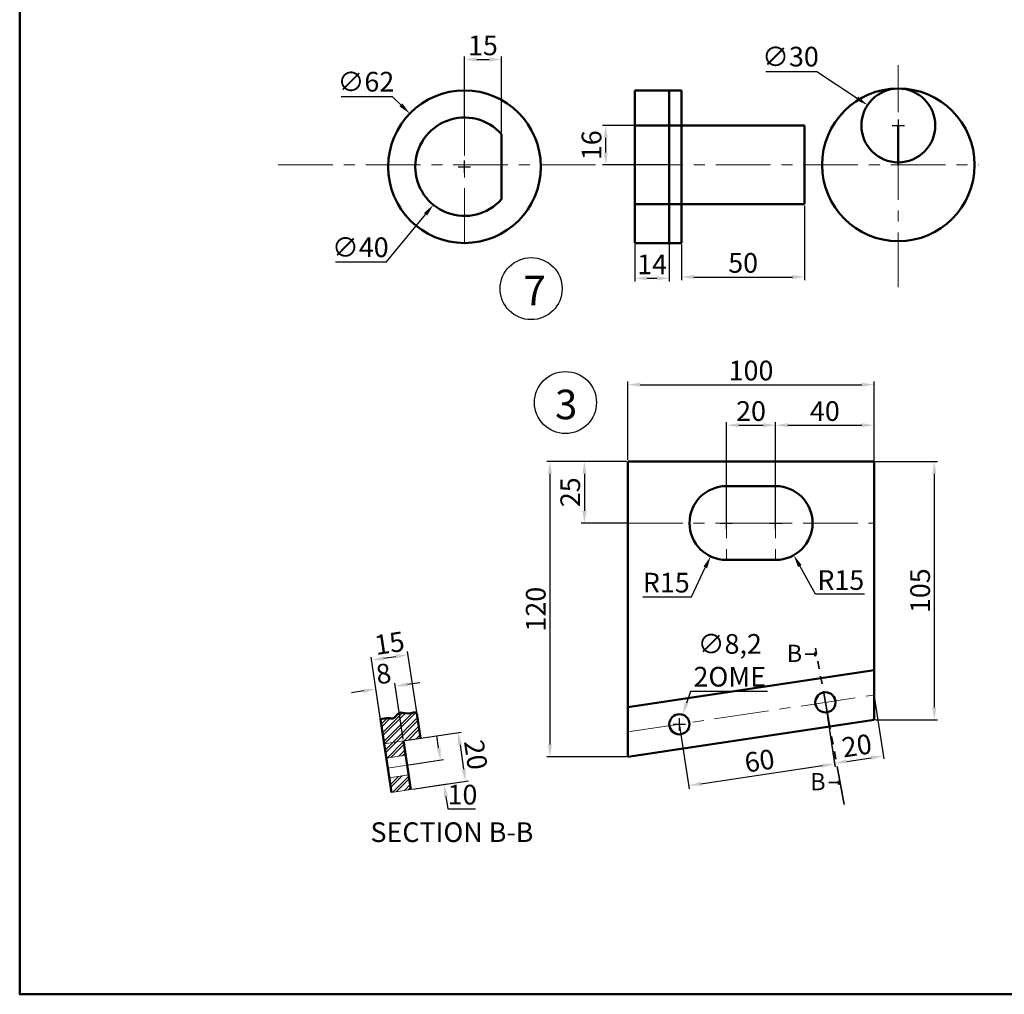
# Model space of a CAD drawing. Units: millimetres. Extents: x -749 to 333, y -22 to 680.
# Tile 1 of 4: x -749 to -349, y -22 to 374. Entities that reach past the tile are written whole.
import ezdxf

# ---------------------------------------------------------------- set-up
doc = ezdxf.new("R2010")
doc.units = ezdxf.units.MM
doc.header["$LTSCALE"] = 0.7
doc.linetypes.add('CENTER', pattern=[50.8, 31.75, -6.35, 6.35, -6.35])
doc.linetypes.add('PHANTOM', pattern=[63.5, 31.75, -6.35, 6.35, -6.35, 6.35, -6.35])
for name, color, linetype, lineweight in [('M-CNTR', 1, 'CENTER', 18), ('M-DIMS', 2, 'Continuous', 25), ('M-HATC', 8, 'Continuous', 18), ('M-OUTL', 7, 'Continuous', 50), ('M-SECT', 6, 'PHANTOM', 35), ('M-TEXT', 3, 'Continuous', 25), ('M-TTLB', 7, 'Continuous', 50)]:
    doc.layers.add(name, color=color, linetype=linetype, lineweight=lineweight)
doc.styles.get("Standard").update_dxf_attribs({"font": 'arial.ttf'})
doc.dimstyles.new('ISO-25', dxfattribs={"dimtxt": 8, "dimasz": 5, "dimexe": 1.25, "dimexo": 0.625, "dimtad": 1, "dimtoh": 1, "dimtxsty": 'Standard', "dimcen": 2.5, "dimadec": 0, "dimazin": 0, "dimtfac": 1, "dimtofl": 0, "dimtmove": 0, "dimatfit": 3, "dimfxl": 1, "dimarcsym": 0})

# ---------------------------------------------------------------- blocks, each defined once
blk = doc.blocks.new('*D36')
at = {"layer": 'Defpoints', "color": 0, "transparency": 16777216}
for p in [(-590.85, 335.54), (-546.39, 292.33)]:
    blk.add_point(p, dxfattribs=at)
at = {"layer": 'M-DIMS', "color": 0, "lineweight": -2, "transparency": 16777216}
for p, q in [((-618.72, 342.51), (-598.02, 342.51)), ((-598.02, 342.51), (-594.43, 339.03)), ((-568.62, 311.43), (-568.62, 316.43)), ((-571.12, 313.93), (-566.12, 313.93))]:
    blk.add_line(p, q, dxfattribs=at)
at = {"layer": 'M-DIMS', "color": 0, "transparency": 16777216}
blk.add_solid([(-593.85, 339.62), (-595.01, 338.43), (-590.85, 335.54)], dxfattribs=at)
at = {"layer": 'M-DIMS', "color": 0, "transparency": 16777216, "insert": (-608.68, 347.44), "char_height": 8, "attachment_point": 5}
blk.add_mtext('∅62', dxfattribs=at)
blk = doc.blocks.new('*D37')
at = {"layer": 'Defpoints', "color": 0, "transparency": 16777216}
for p in [(-555.96, 329.42), (-581.28, 298.45)]:
    blk.add_point(p, dxfattribs=at)
at = {"layer": 'M-DIMS', "color": 0, "lineweight": -2, "transparency": 16777216}
for p, q in [((-568.62, 311.43), (-568.62, 316.43)), ((-571.12, 313.93), (-566.12, 313.93)), ((-600.26, 275.24), (-584.44, 294.58)), ((-621.02, 275.24), (-600.26, 275.24))]:
    blk.add_line(p, q, dxfattribs=at)
at = {"layer": 'M-DIMS', "color": 0, "transparency": 16777216}
blk.add_solid([(-585.09, 295.11), (-583.79, 294.05), (-581.28, 298.45)], dxfattribs=at)
at = {"layer": 'M-DIMS', "color": 0, "transparency": 16777216, "insert": (-610.95, 280.17), "char_height": 8, "attachment_point": 5}
blk.add_mtext('∅40', dxfattribs=at)
blk = doc.blocks.new('*D38')
at = {"layer": 'Defpoints', "color": 0, "transparency": 16777216}
for p in [(-404.82, 338.98), (-379.83, 322.39)]:
    blk.add_point(p, dxfattribs=at)
at = {"layer": 'M-DIMS', "color": 0, "lineweight": -2, "transparency": 16777216}
for p, q in [((-446.23, 352.68), (-425.47, 352.68)), ((-425.47, 352.68), (-408.99, 341.74)), ((-392.32, 328.18), (-392.32, 333.18)), ((-394.82, 330.68), (-389.82, 330.68))]:
    blk.add_line(p, q, dxfattribs=at)
at = {"layer": 'M-DIMS', "color": 0, "transparency": 16777216}
blk.add_solid([(-408.53, 342.44), (-409.45, 341.05), (-404.82, 338.98)], dxfattribs=at)
at = {"layer": 'M-DIMS', "color": 0, "transparency": 16777216, "insert": (-436.16, 357.62), "char_height": 8, "attachment_point": 5}
blk.add_mtext('∅30', dxfattribs=at)
blk = doc.blocks.new('*D39')
at = {"layer": 'Defpoints', "color": 0, "transparency": 16777216}
for p in [(-511.24, 330.68), (-485.39, 330.68), (-485.39, 314.68)]:
    blk.add_point(p, dxfattribs=at)
at = {"layer": 'M-DIMS', "color": 0, "lineweight": -2, "transparency": 16777216}
for p, q in [((-486.01, 330.68), (-512.49, 330.68)), ((-511.24, 319.68), (-511.24, 325.68)), ((-486.01, 314.68), (-512.49, 314.68))]:
    blk.add_line(p, q, dxfattribs=at)
at = {"layer": 'M-DIMS', "color": 0, "transparency": 16777216}
for points in [[(-512.07, 325.68), (-510.4, 325.68), (-511.24, 330.68)], [(-512.07, 319.68), (-510.4, 319.68), (-511.24, 314.68)]]:
    blk.add_solid(points, dxfattribs=at)
at = {"layer": 'M-DIMS', "color": 0, "transparency": 16777216, "insert": (-515.95, 322.68), "char_height": 8, "attachment_point": 5, "rotation": 90}
blk.add_mtext('16', dxfattribs=at)
blk = doc.blocks.new('*D40')
at = {"layer": 'Defpoints', "color": 0, "transparency": 16777216}
for p in [(-499.39, 282.93), (-485.39, 282.93), (-485.39, 268.59)]:
    blk.add_point(p, dxfattribs=at)
at = {"layer": 'M-DIMS', "color": 0, "lineweight": -2, "transparency": 16777216}
for p, q in [((-499.39, 282.31), (-499.39, 267.34)), ((-485.39, 282.31), (-485.39, 267.34)), ((-494.39, 268.59), (-490.39, 268.59))]:
    blk.add_line(p, q, dxfattribs=at)
at = {"layer": 'M-DIMS', "color": 0, "transparency": 16777216}
for points in [[(-494.39, 269.42), (-494.39, 267.76), (-499.39, 268.59)], [(-490.39, 269.42), (-490.39, 267.76), (-485.39, 268.59)]]:
    blk.add_solid(points, dxfattribs=at)
at = {"layer": 'M-DIMS', "color": 0, "transparency": 16777216, "insert": (-492.39, 273.23), "char_height": 8, "attachment_point": 5}
blk.add_mtext('14', dxfattribs=at)
blk = doc.blocks.new('*D41')
at = {"layer": 'Defpoints', "color": 0, "transparency": 16777216}
for p in [(-430.39, 298.68), (-480.39, 282.93), (-430.39, 269.12)]:
    blk.add_point(p, dxfattribs=at)
at = {"layer": 'M-DIMS', "color": 0, "lineweight": -2, "transparency": 16777216}
for p, q in [((-430.39, 298.06), (-430.39, 267.87)), ((-480.39, 282.31), (-480.39, 267.87)), ((-475.39, 269.12), (-435.39, 269.12))]:
    blk.add_line(p, q, dxfattribs=at)
at = {"layer": 'M-DIMS', "color": 0, "transparency": 16777216}
for points in [[(-475.39, 269.95), (-475.39, 268.29), (-480.39, 269.12)], [(-435.39, 269.95), (-435.39, 268.29), (-430.39, 269.12)]]:
    blk.add_solid(points, dxfattribs=at)
at = {"layer": 'M-DIMS', "color": 0, "transparency": 16777216, "insert": (-455.39, 273.83), "char_height": 8, "attachment_point": 5}
blk.add_mtext('50', dxfattribs=at)
blk = doc.blocks.new('*D42')
at = {"layer": 'Defpoints', "color": 0, "transparency": 16777216}
for p in [(-553.62, 357.49), (-568.62, 333.93), (-553.62, 327.16)]:
    blk.add_point(p, dxfattribs=at)
at = {"layer": 'M-DIMS', "color": 0, "lineweight": -2, "transparency": 16777216}
for p, q in [((-568.62, 334.56), (-568.62, 358.74)), ((-563.62, 357.49), (-558.62, 357.49)), ((-553.62, 327.79), (-553.62, 358.74))]:
    blk.add_line(p, q, dxfattribs=at)
at = {"layer": 'M-DIMS', "color": 0, "transparency": 16777216}
for points in [[(-563.62, 358.32), (-563.62, 356.65), (-568.62, 357.49)], [(-558.62, 358.32), (-558.62, 356.65), (-553.62, 357.49)]]:
    blk.add_solid(points, dxfattribs=at)
at = {"layer": 'M-DIMS', "color": 0, "transparency": 16777216, "insert": (-561.12, 362.19), "char_height": 8, "attachment_point": 5}
blk.add_mtext('15', dxfattribs=at)
blk = doc.blocks.new('*D66')
at = {"layer": 'Defpoints', "color": 0, "transparency": 16777216}
for p in [(-402.18, 225.38), (-502.18, 194.18), (-402.18, 194.18)]:
    blk.add_point(p, dxfattribs=at)
at = {"layer": 'M-DIMS', "color": 0, "lineweight": -2, "transparency": 16777216}
for p, q in [((-502.18, 194.8), (-502.18, 226.63)), ((-497.18, 225.38), (-407.18, 225.38)), ((-402.18, 194.8), (-402.18, 226.63))]:
    blk.add_line(p, q, dxfattribs=at)
at = {"layer": 'M-DIMS', "color": 0, "transparency": 16777216}
for points in [[(-497.18, 226.22), (-497.18, 224.55), (-502.18, 225.38)], [(-407.18, 226.22), (-407.18, 224.55), (-402.18, 225.38)]]:
    blk.add_solid(points, dxfattribs=at)
at = {"layer": 'M-DIMS', "color": 0, "transparency": 16777216, "insert": (-452.18, 230.09), "char_height": 8, "attachment_point": 5}
blk.add_mtext('100', dxfattribs=at)
blk = doc.blocks.new('*D67')
at = {"layer": 'Defpoints', "color": 0, "transparency": 16777216}
for p in [(-402.18, 194.18), (-402.18, 89.18), (-377.71, 89.18)]:
    blk.add_point(p, dxfattribs=at)
at = {"layer": 'M-DIMS', "color": 0, "lineweight": -2, "transparency": 16777216}
for p, q in [((-401.55, 194.18), (-376.46, 194.18)), ((-377.71, 189.18), (-377.71, 94.18)), ((-401.55, 89.18), (-376.46, 89.18))]:
    blk.add_line(p, q, dxfattribs=at)
at = {"layer": 'M-DIMS', "color": 0, "transparency": 16777216}
for points in [[(-378.54, 189.18), (-376.87, 189.18), (-377.71, 194.18)], [(-378.54, 94.18), (-376.87, 94.18), (-377.71, 89.18)]]:
    blk.add_solid(points, dxfattribs=at)
at = {"layer": 'M-DIMS', "color": 0, "transparency": 16777216, "insert": (-382.42, 141.68), "char_height": 8, "attachment_point": 5, "rotation": 90}
blk.add_mtext('105', dxfattribs=at)
blk = doc.blocks.new('*D68')
at = {"layer": 'Defpoints', "color": 0, "transparency": 16777216}
for p in [(-442.18, 208.92), (-462.18, 169.18), (-442.18, 169.18)]:
    blk.add_point(p, dxfattribs=at)
at = {"layer": 'M-DIMS', "color": 0, "lineweight": -2, "transparency": 16777216}
for p, q in [((-462.18, 169.8), (-462.18, 210.17)), ((-457.18, 208.92), (-447.18, 208.92)), ((-442.18, 169.8), (-442.18, 210.17))]:
    blk.add_line(p, q, dxfattribs=at)
at = {"layer": 'M-DIMS', "color": 0, "transparency": 16777216}
for points in [[(-457.18, 209.75), (-457.18, 208.08), (-462.18, 208.92)], [(-447.18, 209.75), (-447.18, 208.08), (-442.18, 208.92)]]:
    blk.add_solid(points, dxfattribs=at)
at = {"layer": 'M-DIMS', "color": 0, "transparency": 16777216, "insert": (-452.18, 213.63), "char_height": 8, "attachment_point": 5}
blk.add_mtext('20', dxfattribs=at)
blk = doc.blocks.new('*D69')
at = {"layer": 'Defpoints', "color": 0, "transparency": 16777216}
for p in [(-502.18, 194.18), (-519.89, 169.18), (-502.18, 169.18)]:
    blk.add_point(p, dxfattribs=at)
at = {"layer": 'M-DIMS', "color": 0, "lineweight": -2, "transparency": 16777216}
for p, q in [((-502.8, 194.18), (-521.14, 194.18)), ((-519.89, 189.18), (-519.89, 174.18)), ((-502.8, 169.18), (-521.14, 169.18))]:
    blk.add_line(p, q, dxfattribs=at)
at = {"layer": 'M-DIMS', "color": 0, "transparency": 16777216}
for points in [[(-520.72, 189.18), (-519.05, 189.18), (-519.89, 194.18)], [(-520.72, 174.18), (-519.05, 174.18), (-519.89, 169.18)]]:
    blk.add_solid(points, dxfattribs=at)
at = {"layer": 'M-DIMS', "color": 0, "transparency": 16777216, "insert": (-524.6, 181.68), "char_height": 8, "attachment_point": 5, "rotation": 90}
blk.add_mtext('25', dxfattribs=at)
blk = doc.blocks.new('*D70')
at = {"layer": 'Defpoints', "color": 0, "transparency": 16777216}
for p in [(-421.96, 96.32), (-481.29, 87.42), (-418.21, 71.38)]:
    blk.add_point(p, dxfattribs=at)
at = {"layer": 'M-DIMS', "color": 0, "lineweight": -2, "transparency": 16777216}
for p, q in [((-421.86, 95.7), (-418.03, 70.14)), ((-481.2, 86.8), (-477.37, 61.24)), ((-472.61, 63.22), (-423.16, 70.64))]:
    blk.add_line(p, q, dxfattribs=at)
at = {"layer": 'M-DIMS', "color": 0, "transparency": 16777216}
for points in [[(-423.28, 71.46), (-423.04, 69.81), (-418.21, 71.38)], [(-472.73, 64.04), (-472.48, 62.39), (-477.55, 62.48)]]:
    blk.add_solid(points, dxfattribs=at)
at = {"layer": 'M-DIMS', "color": 0, "transparency": 16777216, "insert": (-448.58, 71.58), "char_height": 8, "attachment_point": 5, "rotation": 8.5308}
blk.add_mtext('60', dxfattribs=at)
blk = doc.blocks.new('*D71')
at = {"layer": 'Defpoints', "color": 0, "transparency": 16777216}
for p in [(-421.96, 96.32), (-402.18, 99.29), (-398.47, 74.54)]:
    blk.add_point(p, dxfattribs=at)
at = {"layer": 'M-DIMS', "color": 0, "lineweight": -2, "transparency": 16777216}
for p, q in [((-402.08, 98.67), (-398.28, 73.31)), ((-421.86, 95.7), (-418.06, 70.34)), ((-413.3, 72.32), (-403.41, 73.8))]:
    blk.add_line(p, q, dxfattribs=at)
at = {"layer": 'M-DIMS', "color": 0, "transparency": 16777216}
for points in [[(-413.42, 73.14), (-413.18, 71.49), (-418.24, 71.57)], [(-403.53, 74.62), (-403.29, 72.98), (-398.47, 74.54)]]:
    blk.add_solid(points, dxfattribs=at)
at = {"layer": 'M-DIMS', "color": 0, "transparency": 16777216, "insert": (-409.05, 77.72), "char_height": 8, "attachment_point": 5, "rotation": 8.5308}
blk.add_mtext('20', dxfattribs=at)
blk = doc.blocks.new('*D72')
at = {"layer": 'Defpoints', "color": 0, "transparency": 16777216}
for p in [(-502.18, 194.18), (-533.91, 74.18), (-502.18, 74.18)]:
    blk.add_point(p, dxfattribs=at)
at = {"layer": 'M-DIMS', "color": 0, "lineweight": -2, "transparency": 16777216}
for p, q in [((-502.8, 194.18), (-535.16, 194.18)), ((-533.91, 189.18), (-533.91, 79.18)), ((-502.8, 74.18), (-535.16, 74.18))]:
    blk.add_line(p, q, dxfattribs=at)
at = {"layer": 'M-DIMS', "color": 0, "transparency": 16777216}
for points in [[(-534.75, 189.18), (-533.08, 189.18), (-533.91, 194.18)], [(-534.75, 79.18), (-533.08, 79.18), (-533.91, 74.18)]]:
    blk.add_solid(points, dxfattribs=at)
at = {"layer": 'M-DIMS', "color": 0, "transparency": 16777216, "insert": (-538.62, 134.18), "char_height": 8, "attachment_point": 5, "rotation": 90}
blk.add_mtext('120', dxfattribs=at)
blk = doc.blocks.new('*D73')
at = {"layer": 'Defpoints', "color": 0, "transparency": 16777216}
for p in [(-479.99, 91.31), (-482.59, 83.53)]:
    blk.add_point(p, dxfattribs=at)
at = {"layer": 'M-DIMS', "color": 0, "lineweight": -2, "transparency": 16777216}
for p, q in [((-476.81, 100.79), (-478.4, 96.05)), ((-445.44, 100.79), (-476.81, 100.79)), ((-481.29, 84.92), (-481.29, 89.92)), ((-483.79, 87.42), (-478.79, 87.42))]:
    blk.add_line(p, q, dxfattribs=at)
at = {"layer": 'M-DIMS', "color": 0, "transparency": 16777216}
blk.add_solid([(-479.19, 96.31), (-477.61, 95.78), (-479.99, 91.31)], dxfattribs=at)
at = {"layer": 'M-DIMS', "color": 0, "transparency": 16777216, "insert": (-460.82, 112.37), "char_height": 8, "attachment_point": 5}
blk.add_mtext('∅8,2\\P2OME', dxfattribs=at)
blk = doc.blocks.new('*D74')
at = {"layer": 'Defpoints', "color": 0, "transparency": 16777216}
for p in [(-462.18, 169.18), (-468.61, 155.63)]:
    blk.add_point(p, dxfattribs=at)
at = {"layer": 'M-DIMS', "color": 0, "lineweight": -2, "transparency": 16777216}
for p, q in [((-464.68, 169.18), (-459.68, 169.18)), ((-462.18, 166.68), (-462.18, 171.68)), ((-476.41, 139.22), (-470.76, 151.11)), ((-496.21, 139.22), (-476.41, 139.22))]:
    blk.add_line(p, q, dxfattribs=at)
at = {"layer": 'M-DIMS', "color": 0, "transparency": 16777216}
blk.add_solid([(-471.51, 151.47), (-470.01, 150.75), (-468.61, 155.63)], dxfattribs=at)
at = {"layer": 'M-DIMS', "color": 0, "transparency": 16777216, "insert": (-486.62, 143.92), "char_height": 8, "attachment_point": 5}
blk.add_mtext('R15', dxfattribs=at)
blk = doc.blocks.new('*D75')
at = {"layer": 'Defpoints', "color": 0, "transparency": 16777216}
for p in [(-442.18, 169.18), (-434.83, 156.1)]:
    blk.add_point(p, dxfattribs=at)
at = {"layer": 'M-DIMS', "color": 0, "lineweight": -2, "transparency": 16777216}
for p, q in [((-444.68, 169.18), (-439.68, 169.18)), ((-442.18, 166.68), (-442.18, 171.68)), ((-425.92, 140.26), (-432.38, 151.74)), ((-406.12, 140.26), (-425.92, 140.26))]:
    blk.add_line(p, q, dxfattribs=at)
at = {"layer": 'M-DIMS', "color": 0, "transparency": 16777216}
blk.add_solid([(-431.65, 152.15), (-433.1, 151.33), (-434.83, 156.1)], dxfattribs=at)
at = {"layer": 'M-DIMS', "color": 0, "transparency": 16777216, "insert": (-415.71, 144.97), "char_height": 8, "attachment_point": 5}
blk.add_mtext('R15', dxfattribs=at)
blk = doc.blocks.new('*D76')
at = {"layer": 'Defpoints', "color": 0, "transparency": 16777216}
for p in [(-593.38, 80.72), (-568.22, 64.27), (-590.41, 60.94)]:
    blk.add_point(p, dxfattribs=at)
at = {"layer": 'M-DIMS', "color": 0, "lineweight": -2, "transparency": 16777216}
for p, q in [((-592.76, 80.81), (-569.95, 84.23)), ((-570.44, 79.1), (-568.96, 69.22)), ((-589.79, 61.03), (-566.98, 64.46))]:
    blk.add_line(p, q, dxfattribs=at)
at = {"layer": 'M-DIMS', "color": 0, "transparency": 16777216}
for points in [[(-569.62, 79.23), (-571.27, 78.98), (-571.18, 84.05)], [(-568.13, 69.34), (-569.78, 69.09), (-568.22, 64.27)]]:
    blk.add_solid(points, dxfattribs=at)
at = {"layer": 'M-DIMS', "color": 0, "transparency": 16777216, "insert": (-565.04, 74.86), "char_height": 8, "attachment_point": 5, "rotation": 278.5308}
blk.add_mtext('20', dxfattribs=at)
blk = doc.blocks.new('*D77')
at = {"layer": 'Defpoints', "color": 0, "transparency": 16777216}
for p in [(-591.89, 70.83), (-590.41, 60.94), (-576.89, 62.97)]:
    blk.add_point(p, dxfattribs=at)
at = {"layer": 'M-DIMS', "color": 0, "lineweight": -2, "transparency": 16777216}
for p, q in [((-579.11, 77.8), (-579.85, 82.75)), ((-591.28, 70.92), (-577.13, 73.04)), ((-589.79, 61.03), (-575.65, 63.16)), ((-576.15, 58.03), (-575.4, 53.08)), ((-575.4, 53.08), (-564.1, 53.08))]:
    blk.add_line(p, q, dxfattribs=at)
at = {"layer": 'M-DIMS', "color": 0, "transparency": 16777216}
for points in [[(-578.29, 77.93), (-579.94, 77.68), (-578.37, 72.86)], [(-575.32, 58.15), (-576.97, 57.9), (-576.89, 62.97)]]:
    blk.add_solid(points, dxfattribs=at)
at = {"layer": 'M-DIMS', "color": 0, "transparency": 16777216, "insert": (-569.44, 57.79), "char_height": 8, "attachment_point": 5}
blk.add_mtext('10', dxfattribs=at)
blk = doc.blocks.new('*D78')
at = {"layer": 'Defpoints', "color": 0, "transparency": 16777216}
for p in [(-591.55, 115.71), (-602.77, 89.44), (-587.94, 91.66)]:
    blk.add_point(p, dxfattribs=at)
at = {"layer": 'M-DIMS', "color": 0, "lineweight": -2, "transparency": 16777216}
for p, q in [((-588.03, 92.28), (-591.73, 116.95)), ((-602.87, 90.06), (-606.57, 114.72)), ((-601.44, 114.23), (-596.49, 114.97))]:
    blk.add_line(p, q, dxfattribs=at)
at = {"layer": 'M-DIMS', "color": 0, "transparency": 16777216}
for points in [[(-601.56, 115.05), (-601.31, 113.4), (-606.38, 113.49)], [(-596.62, 115.79), (-596.37, 114.15), (-591.55, 115.71)]]:
    blk.add_solid(points, dxfattribs=at)
at = {"layer": 'M-DIMS', "color": 0, "transparency": 16777216, "insert": (-598.95, 119.36), "char_height": 8, "attachment_point": 5, "rotation": 8.5308}
blk.add_mtext('15', dxfattribs=at)
blk = doc.blocks.new('*D79')
at = {"layer": 'Defpoints', "color": 0, "transparency": 16777216}
for p in [(-596.71, 102.91), (-593.38, 80.72), (-601.29, 79.53)]:
    blk.add_point(p, dxfattribs=at)
at = {"layer": 'M-DIMS', "color": 0, "lineweight": -2, "transparency": 16777216}
for p, q in [((-593.47, 81.34), (-596.89, 104.14)), ((-591.76, 103.65), (-586.82, 104.39)), ((-609.56, 100.98), (-614.51, 100.24)), ((-601.38, 80.15), (-604.8, 102.96))]:
    blk.add_line(p, q, dxfattribs=at)
at = {"layer": 'M-DIMS', "color": 0, "transparency": 16777216}
for points in [[(-591.88, 104.47), (-591.64, 102.83), (-596.71, 102.91)], [(-609.69, 101.8), (-609.44, 100.16), (-604.62, 101.72)]]:
    blk.add_solid(points, dxfattribs=at)
at = {"layer": 'M-DIMS', "color": 0, "transparency": 16777216, "insert": (-601.36, 106.97), "char_height": 8, "attachment_point": 5, "rotation": 8.5308}
blk.add_mtext('8', dxfattribs=at)
blk = doc.blocks.new('*D88')
at = {"layer": 'Defpoints', "color": 0, "ltscale": 0.7, "transparency": 16777216}
for p in [(-402.18, 208.92), (-402.18, 178.12), (-442.18, 169.18)]:
    blk.add_point(p, dxfattribs=at)
at = {"layer": 'M-DIMS', "color": 0, "lineweight": -2, "ltscale": 0.7, "transparency": 16777216}
for p, q in [((-442.18, 169.8), (-442.18, 210.17)), ((-437.18, 208.92), (-407.18, 208.92)), ((-402.18, 178.75), (-402.18, 210.17))]:
    blk.add_line(p, q, dxfattribs=at)
at = {"layer": 'M-DIMS', "color": 0, "ltscale": 0.7, "transparency": 16777216}
for points in [[(-437.18, 209.75), (-437.18, 208.08), (-442.18, 208.92)], [(-407.18, 209.75), (-407.18, 208.08), (-402.18, 208.92)]]:
    blk.add_solid(points, dxfattribs=at)
at = {"layer": 'M-DIMS', "color": 0, "ltscale": 0.7, "transparency": 16777216, "insert": (-422.18, 213.63), "char_height": 8, "attachment_point": 5}
blk.add_mtext('40', dxfattribs=at)

msp = doc.modelspace()

# ---------------------------------------------------------------- hatches: boundary and pattern name
at = {"layer": 'M-HATC', "ltscale": 0.7}
h = msp.add_hatch(dxfattribs=at)
h.set_pattern_fill('ANSI32', color=256, scale=0.3)
h.set_pattern_definition([(45, (-3477.0897, -507.9452), (-2.0205576, 2.0205576), []), (45, (-3475.7427, -507.9452), (-2.0205576, 2.0205576), [])])
edge = h.paths.add_edge_path()
edge.add_spline(control_points=[(-587.97, 91.861), (-588.348, 92.607), (-591.937, 91.134), (-595.435, 93.056), (-597.003, 89.411), (-599.981, 90.2), (-601.71, 89.728), (-602.775, 89.438)], knot_values=[0, 0, 0, 0, 3.4976081, 7.5126071, 10.2409894, 12.3136778, 15.6403307, 15.6403307, 15.6403307, 15.6403307], degree=3, periodic=0)
edge.add_line((-602.775, 89.438), (-601.289, 79.533))
edge.add_line((-601.289, 79.533), (-586.455, 81.759))
edge.add_line((-586.455, 81.759), (-587.97, 91.861))
h.paths.add_polyline_path([(-593.378, 80.72), (-601.289, 79.533), (-600.408, 73.657), (-592.496, 74.844)])
h.paths.add_polyline_path([(-591.293, 66.823), (-599.205, 65.637), (-598.322, 59.755), (-590.411, 60.941)])

# ---------------------------------------------------------------- linework, layer by layer
at = {"layer": 'M-CNTR'}
for p, q in [((-392.323, 264.979), (-392.323, 355.252)), ((-568.616, 282.934), (-568.616, 344.934)), ((-644.284, 314.684), (-537.625, 314.684)), ((-537.625, 314.684), (-359.786, 314.684)), ((-462.178, 194.176), (-462.178, 154.176)), ((-442.178, 194.176), (-442.178, 154.176)), ((-502.178, 169.176), (-402.178, 169.176)), ((-502.178, 84.288), (-402.178, 99.288)), ((-402.178, 89.176), (-400.694, 89.399)), ((-601.289, 79.533), (-586.455, 81.759)), ((-600.408, 73.657), (-592.496, 74.844)), ((-599.806, 69.644), (-584.972, 71.869)), ((-599.205, 65.637), (-591.293, 66.823)), ((-598.322, 59.755), (-590.411, 60.941))]:
    msp.add_line(p, q, dxfattribs=at)
at = {"layer": 'M-OUTL'}
for p, q in [((-499.387, 282.934), (-499.387, 344.934)), ((-499.387, 344.934), (-485.387, 344.934)), ((-485.387, 344.934), (-485.387, 282.934)), ((-480.387, 344.934), (-485.387, 344.934)), ((-480.387, 344.934), (-480.387, 282.934)), ((-499.387, 330.684), (-430.387, 330.684)), ((-430.387, 298.684), (-430.387, 330.684)), ((-553.617, 300.703), (-553.617, 327.164)), ((-499.387, 298.684), (-430.387, 298.684)), ((-485.387, 282.934), (-499.387, 282.934)), ((-499.387, 282.934), (-480.387, 282.934)), ((-502.178, 194.176), (-402.178, 194.176)), ((-502.178, 194.176), (-502.178, 74.176)), ((-402.178, 194.176), (-402.178, 89.176)), ((-462.178, 184.176), (-442.178, 184.176)), ((-462.178, 154.176), (-442.178, 154.176)), ((-502.178, 94.4), (-402.178, 109.4)), ((-601.289, 79.533), (-602.775, 89.438)), ((-586.455, 81.759), (-587.97, 91.861)), ((-502.178, 74.176), (-402.178, 89.176)), ((-593.378, 80.72), (-590.411, 60.941)), ((-601.289, 79.533), (-598.322, 59.755))]:
    msp.add_line(p, q, dxfattribs=at)
at = {"layer": 'M-OUTL', "ltscale": 0.7}
msp.add_line((-392.323, 314.684), (-392.323, 330.684), dxfattribs=at)
at = {"layer": 'M-OUTL'}
for centre, radius in [((-568.616, 313.934), 31), ((-392.323, 314.684), 31), ((-392.323, 330.684), 15), ((-421.956, 96.321), 4.1), ((-481.292, 87.421), 4.1), ((-481.292, 87.421), 4.1)]:
    msp.add_circle(centre, radius, dxfattribs=at)
for centre, radius, start, end in [((-568.616, 313.934), 20, 41.41641, 318.58359), ((-462.178, 169.176), 15, 90, 270), ((-442.178, 169.176), 15, 270, 90)]:
    msp.add_arc(centre, radius, start, end, dxfattribs=at)
msp.add_open_spline([(-602.775, 89.438), (-601.71, 89.728), (-599.981, 90.2), (-597.003, 89.411), (-595.435, 93.056), (-591.937, 91.134), (-588.348, 92.607), (-587.97, 91.861)], degree=3, knots=[0, 0, 0, 0, 3.3266529, 5.3993413, 8.1277235, 12.1427226, 15.6403307, 15.6403307, 15.6403307, 15.6403307], dxfattribs=at)
at = {"layer": 'M-SECT', "ltscale": 0.7}
for p, q in [((-425.526, 115.851), (-426.233, 116.558)), ((-426.233, 116.558), (-426.233, 115.144)), ((-414.383, 54.891), (-425.971, 118.286)), ((-430.118, 115.853), (-425.526, 115.851)), ((-425.526, 115.851), (-426.233, 115.144)), ((-415.995, 63.711), (-416.702, 64.418)), ((-416.702, 64.418), (-416.702, 63.004)), ((-420.588, 63.713), (-415.995, 63.711)), ((-415.995, 63.711), (-416.702, 63.004))]:
    msp.add_line(p, q, dxfattribs=at)
at = {"layer": 'M-TEXT'}
for centre in [(-541.538, 264.395), (-527.586, 218.129)]:
    msp.add_circle(centre, 12.598, dxfattribs=at)
at = {"layer": 'M-TTLB', "ltscale": 0.7}
msp.add_lwpolyline([(-749.362, 679.91), (332.782, 679.91), (332.782, -22.287), (-749.362, -22.287)], close=True, dxfattribs=at)

# ---------------------------------------------------------------- texts
at = {"layer": 'M-TEXT', "attachment_point": 1}
for s, width, insert, char_height in [('7', 30.10277, (-544.685, 269.614), 12), ('\\pxql;3', 12, (-531.84, 223.348), 12), ('SECTION B-B', 95.89335, (-606.818, 47.575), 8)]:
    msp.add_mtext_dynamic_manual_height_columns(s, width=width, gutter_width=12.5, heights=[0], dxfattribs=dict(at, insert=insert, char_height=char_height))
at = {"layer": 'M-TEXT', "ltscale": 0.7, "char_height": 7, "attachment_point": 1}
for insert in [(-437.678, 119.727), (-428.148, 67.587)]:
    msp.add_mtext_dynamic_manual_height_columns('B', width=7.19522, gutter_width=12.5, heights=[0], dxfattribs=dict(at, insert=insert))

# ---------------------------------------------------------------- dimensions: what is measured, and where the dimension line sits
at = {"layer": 'M-DIMS'}
for base, p1, p2, picture, middle in [((-553.617, 357.485), (-568.616, 333.934), (-553.617, 327.164), '*D42', (-561.117, 362.195)), ((-430.387, 269.121), (-480.387, 282.934), (-430.387, 298.684), '*D41', (-455.387, 273.831)), ((-485.387, 268.591), (-499.387, 282.934), (-485.387, 282.934), '*D40', (-492.387, 273.232)), ((-402.178, 225.383), (-502.178, 194.176), (-402.178, 194.176), '*D66', (-452.178, 230.093)), ((-442.178, 208.916), (-462.178, 169.176), (-442.178, 169.176), '*D68', (-452.178, 213.626))]:
    dim = msp.add_linear_dim(base=base, p1=p1, p2=p2, dimstyle='ISO-25', override={"dimclrd": 0, "dimclre": 0, "dimclrt": 0}, dxfattribs=at)
    dim.commit()
    dim.dimension.update_dxf_attribs({"geometry": picture, "text_midpoint": middle})
for p1, p2, picture, middle in [((-379.825, 322.389), (-404.821, 338.979), '*D38', (-436.161, 352.683)), ((-555.956, 329.417), (-581.275, 298.45), '*D37', (-610.949, 275.235))]:
    dim = msp.add_diameter_dim_2p(p1=p1, p2=p2, dimstyle='ISO-25', override={"dimclrd": 0, "dimclre": 0, "dimclrt": 0}, dxfattribs=at)
    dim.commit()
    dim.dimension.update_dxf_attribs({"geometry": picture, "text_midpoint": middle, "dimtype": 163})
dim = msp.add_diameter_dim_2p(p1=(-546.386, 292.328), p2=(-590.846, 335.54), dimstyle='ISO-25', override={"dimclrd": 0, "dimclre": 0, "dimclrt": 0}, dxfattribs=at)
dim.commit()
dim.dimension.update_dxf_attribs({"geometry": '*D36', "text_midpoint": (-608.682, 347.443)})
for base, p1, p2, picture, middle in [((-511.237, 330.684), (-485.387, 314.684), (-485.387, 330.684), '*D39', (-515.947, 322.684)), ((-533.915, 74.176), (-502.178, 194.176), (-502.178, 74.176), '*D72', (-538.624, 134.176)), ((-519.887, 169.176), (-502.178, 194.176), (-502.178, 169.176), '*D69', (-524.596, 181.676)), ((-377.706, 89.176), (-402.178, 194.176), (-402.178, 89.176), '*D67', (-382.415, 141.676))]:
    dim = msp.add_linear_dim(base=base, p1=p1, p2=p2, angle=90, dimstyle='ISO-25', override={"dimclrd": 0, "dimclre": 0, "dimclrt": 0}, dxfattribs=at)
    dim.commit()
    dim.dimension.update_dxf_attribs({"geometry": picture, "text_midpoint": middle})
at = {"layer": 'M-DIMS', "ltscale": 0.7}
dim = msp.add_linear_dim(base=(-402.178, 208.916), p1=(-442.178, 169.176), p2=(-402.178, 178.122), dimstyle='ISO-25', override={"dimclrd": 0, "dimclre": 0, "dimclrt": 0}, dxfattribs=at)
dim.commit()
dim.dimension.update_dxf_attribs({"geometry": '*D88', "text_midpoint": (-422.178, 213.626)})
at = {"layer": 'M-DIMS'}
for center, mpoint, picture, middle in [((-462.178, 169.176), (-468.613, 155.627), '*D74', (-486.622, 143.925)), ((-442.178, 169.176), (-434.827, 156.101), '*D75', (-415.711, 144.972))]:
    dim = msp.add_radius_dim(center=center, mpoint=mpoint, dimstyle='ISO-25', override={"dimclrd": 0, "dimclre": 0, "dimclrt": 0}, dxfattribs=at)
    dim.commit()
    dim.dimension.update_dxf_attribs({"geometry": picture, "text_midpoint": middle})
for base, p1, p2, picture, middle in [((-591.548, 115.712), (-602.775, 89.438), (-587.941, 91.663), '*D78', (-598.255, 114.706)), ((-596.706, 102.908), (-601.289, 79.533), (-593.378, 80.72), '*D79', (-600.662, 102.315))]:
    dim = msp.add_linear_dim(base=base, p1=p1, p2=p2, angle=8.53077, dimstyle='ISO-25', override={"dimclrd": 0, "dimclre": 0, "dimclrt": 0}, dxfattribs=at)
    dim.commit()
    dim.dimension.update_dxf_attribs({"geometry": picture, "text_midpoint": middle, "dimtype": 161})
dim = msp.add_diameter_dim_2p(p1=(-482.595, 83.533), p2=(-479.99, 91.309), text='<>\\P2OME', dimstyle='ISO-25', override={"dimclrd": 0, "dimclre": 0, "dimclrt": 0}, dxfattribs=at)
dim.commit()
dim.dimension.update_dxf_attribs({"geometry": '*D73', "text_midpoint": (-460.816, 112.369)})
for p1, p2, distance, picture, middle in [((-481.292, 87.421), (-421.956, 96.321), -25.224, '*D70', (-448.581, 71.584)), ((-421.956, 96.321), (-402.178, 99.288), -25.024, '*D71', (-409.054, 77.716)), ((-593.378, 80.72), (-590.411, 60.941), 22.442, '*D76', (-565.043, 74.858)), ((-591.894, 70.831), (-590.411, 60.941), 13.674, '*D77', (-569.44, 57.79))]:
    dim = msp.add_aligned_dim(p1=p1, p2=p2, distance=distance, dimstyle='ISO-25', override={"dimclrd": 0, "dimclre": 0, "dimclrt": 0}, dxfattribs=at)
    dim.commit()
    dim.dimension.update_dxf_attribs({"geometry": picture, "text_midpoint": middle})

doc.saveas('drawing.dxf')
